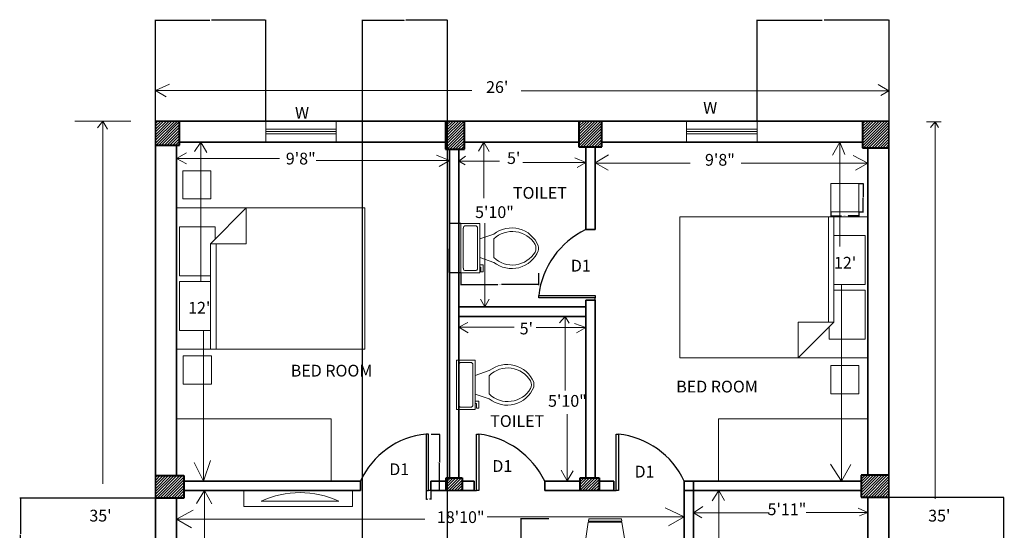
# Model space of a CAD drawing. Units: inches. Extents: x -34 to 385, y -422 to 64.
# Tile 3 of 3: x -34 to 385, y -153 to 64. Entities that reach past the tile are written whole.
import ezdxf

# ---------------------------------------------------------------- set-up
doc = ezdxf.new("R2010")
doc.units = ezdxf.units.IN
doc.header["$MEASUREMENT"] = 0
for name, color, linetype, lineweight in [('A-ANNO-DIMS', 2, 'Continuous', 13), ('A-ANNO-TEXT', 7, 'Continuous', 18), ('A-AREA-IDEN', 7, 'Continuous', 25), ('A-COLS', 1, 'Continuous', 40), ('A-COLS-PATT', 252, 'Continuous', 13), ('A-DOOR', 3, 'Continuous', 25), ('A-FLOR-CASE', 32, 'Continuous', 20), ('A-FLOR-FIXT', 9, 'Continuous', 18), ('A-FURN', 8, 'Continuous', 18), ('A-GLAZ', 4, 'Continuous', 18), ('A-WALL', 7, 'Continuous', 35)]:
    doc.layers.add(name, color=color, linetype=linetype, lineweight=lineweight)
doc.styles.get("Standard").update_dxf_attribs({"font": 'arial.ttf'})
doc.dimstyles.get("Standard").update_dxf_attribs({"dimtxt": 0.18, "dimasz": 0.18, "dimexe": 0.18, "dimexo": 0.0625, "dimgap": 0.09, "dimtad": 0, "dimtih": 1, "dimtoh": 1, "dimdec": 4, "dimzin": 0, "dimdsep": 46, "dimtxsty": 'Standard', "dimcen": 0.09, "dimadec": 0, "dimazin": 0, "dimtfac": 1, "dimtdec": 4, "dimtofl": 0, "dimtmove": 0, "dimatfit": 3, "dimfxl": 1, "dimtolj": 1, "dimtzin": 0, "dimarcsym": 0})

# ---------------------------------------------------------------- blocks, each defined once
blk = doc.blocks.new('Toilet - top')
for p, q in [((9.5, -6), (9.5, -2)), ((-8, -8.5), (-8, -8)), ((-7, -8), (-7, -9.5)), ((-4, -8), (-6, -14)), ((4, -8), (6, -14)), ((-10, -8.5), (-8, -8.5)), ((-10, -9.5), (-10, -8.5)), ((-7, -9.5), (-10, -9.5)), ((4, -14), (-4, -14))]:
    blk.add_line(p, q)
blk.add_lwpolyline([(10.5, -8), (10.5, 0), (-10.5, 0), (-10.5, -8)], close=True)
for points in [[(-9.5, -2), (-9.5, -6)], [(8.5, -1), (-8.5, -1)], [(-8.5, -7), (8.5, -7)]]:
    blk.add_lwpolyline(points)
for centre, radius, start, end in [((-8.62, -1.88), 0.884, 81.8699, 188.1301), ((8.62, -1.88), 0.884, 351.8699, 98.1301), ((-8.62, -6.12), 0.884, 171.8699, 278.1301), ((8.62, -6.12), 0.884, 261.8699, 8.1301), ((3.52, -21.58), 12.17, 141.4691, 247.9714), ((4.2, -21.82), 11.33, 136.3677, 238.9468), ((-3.52, -21.58), 12.17, 292.0284, 38.5307), ((-4.2, -21.82), 11.33, 301.053, 43.6321), ((0, -27.88), 4, 245.7318, 294.2682), ((0, -29), 4, 254.8605, 285.1395)]:
    blk.add_arc(centre, radius, start, end)
blk = doc.blocks.new('Bed - Queen')
for p, q in [((0, -80.00003), (0, 0)), ((0, 0), (59.99999, 0)), ((59.99999, 0), (59.99999, -80.00003)), ((7.99999, -1.2), (28.79998, -1.2)), ((7.99999, -14.4), (7.99999, -1.2)), ((28.79998, -1.2), (28.79998, -14.4)), ((31.19999, -1.2), (51.99999, -1.2)), ((31.19999, -14.4), (31.19999, -1.2)), ((51.99999, -1.2), (51.99999, -16.4)), ((0, -14.4), (44.8, -14.4)), ((59.99999, -29.6), (44.8, -14.4)), ((44.8, -14.4), (44.8, -29.6)), ((51.99999, -16.4), (46.79936, -16.4)), ((44.8, -16.8), (0, -16.8)), ((44.8, -29.6), (59.99999, -29.6)), ((59.99999, -80.00003), (0, -80.00003))]:
    blk.add_line(p, q)
blk = doc.blocks.new('Dining Set - 36 x 72 in.')
for p, q in [((-22.2343, 26.00059), (-23.4847, 17.99762)), ((-22.2304, 26), (-5.7608, 26)), ((-22, 27.5), (-22.1562, 26.50042)), ((-5.8416, 26.5), (-22.1534, 26.5)), ((-22, 27.5), (-6, 27.5)), ((-5.8437, 26.49966), (-6, 27.5)), ((-4.5152, 17.99762), (-5.7655, 25.99926)), ((5.7657, 26.00059), (4.5153, 17.99762)), ((5.7696, 26), (22.2392, 26)), ((6, 27.5), (5.8438, 26.50042)), ((22.1584, 26.5), (5.8466, 26.5)), ((6, 27.5), (22, 27.5)), ((22.1563, 26.49966), (22, 27.5)), ((23.4848, 17.99762), (22.2345, 25.99926)), ((36, 18), (-36, 18)), ((-36, 18), (-36, -18)), ((36, -18), (36, 18)), ((-45.5, 8), (-44.5004, 8.15617)), ((-45.5, 8), (-45.5, -8)), ((-44.5, -8.15843), (-44.5, 8.15338)), ((-44.0006, 8.23428), (-35.9976, 9.48474)), ((-44, 8.23041), (-44, -8.23915)), ((44.0006, 8.23428), (35.9976, 9.48474)), ((44, 8.23041), (44, -8.23915)), ((44.5, -8.15843), (44.5, 8.15338)), ((45.5, 8), (44.5005, 8.15617)), ((45.5, 8), (45.5, -8)), ((-44.4997, -8.15631), (-45.5, -8)), ((-35.9976, -9.48476), (-43.9993, -8.2345)), ((35.9976, -9.48476), (43.9993, -8.2345)), ((44.4997, -8.15631), (45.5, -8)), ((-36, -18), (36, -18)), ((-22.2343, -26.0006), (-23.4847, -17.99762)), ((-4.5152, -17.99762), (-5.7655, -25.99928)), ((5.7657, -26.0006), (4.5153, -17.99762)), ((23.4848, -17.99762), (22.2345, -25.99928)), ((-22.2304, -26), (-5.7608, -26)), ((-22, -27.5), (-22.1562, -26.50044)), ((-5.8416, -26.5), (-22.1534, -26.5)), ((-22, -27.5), (-6, -27.5)), ((-5.8437, -26.49967), (-6, -27.5)), ((5.7696, -26), (22.2392, -26)), ((6, -27.5), (5.8438, -26.50044)), ((22.1584, -26.5), (5.8466, -26.5)), ((6, -27.5), (22, -27.5)), ((22.1563, -26.49967), (22, -27.5))]:
    blk.add_line(p, q)
for points in [[(-36, 15), (-31.1772, 14.97754), (-26.8079, 14.91406), (-22.8538, 14.81543), (-19.276, 14.6875), (-16.0362, 14.53613), (-13.0957, 14.36718), (-10.4159, 14.18652), (-7.9583, 14), (-5.6904, 13.81315), (-3.6035, 13.63021), (-1.6954, 13.45508), (0.0365, 13.29166), (1.5945, 13.14388), (2.9811, 13.01562), (4.1988, 12.9108), (5.25, 12.83333), (6.1393, 12.78613), (6.8802, 12.76823), (7.4883, 12.77767), (7.9792, 12.8125), (8.3685, 12.87077), (8.6719, 12.95052), (8.9049, 13.0498), (9.0833, 13.16666), (9.2205, 13.29899), (9.3216, 13.44401), (9.3895, 13.59879), (9.4271, 13.76041), (9.4373, 13.92594), (9.4232, 14.09245), (9.3875, 14.257), (9.3333, 14.41666), (9.2638, 14.56917), (9.1836, 14.71484), (9.0975, 14.85465), (9.0104, 14.98958), (8.9272, 15.1206), (8.8529, 15.2487), (8.7922, 15.37483), (8.75, 15.5), (8.7305, 15.62467), (8.7344, 15.74739), (8.7617, 15.86621), (8.8125, 15.97916), (8.8867, 16.08431), (8.9844, 16.17968), (9.1055, 16.26334), (9.25, 16.33333), (9.4189, 16.38802), (9.6172, 16.42708), (9.8506, 16.45052), (10.125, 16.45833), (10.4463, 16.45052), (10.8203, 16.42708), (11.2529, 16.38802), (11.75, 16.33333), (12.3184, 16.26318), (12.9694, 16.17838), (13.7151, 16.07991), (14.5677, 15.96875), (15.5395, 15.84586), (16.6426, 15.71224), (17.8893, 15.56884), (19.2917, 15.41666), (20.859, 15.25667), (22.5879, 15.08984), (24.4721, 14.91715), (26.5052, 14.73958), (28.6809, 14.5581), (30.9929, 14.3737), (33.4347, 14.18733), (36, 14)], [(-36, 10), (-28.9766, 10.14274), (-23.1725, 10.20442), (-18.4241, 10.19775), (-14.5677, 10.13541), (-11.4399, 10.03011), (-8.877, 9.89453), (-6.7154, 9.74137), (-4.7917, 9.58333), (-2.9698, 9.43082), (-1.2246, 9.28515), (0.4415, 9.14534), (2.026, 9.01041), (3.5266, 8.87939), (4.9408, 8.7513), (6.266, 8.62516), (7.5, 8.5), (8.6411, 8.37549), (9.6914, 8.2539), (10.6538, 8.13818), (11.5312, 8.03125), (12.3267, 7.93603), (13.043, 7.85547), (13.6831, 7.79248), (14.25, 7.75), (14.7471, 7.7303), (15.1797, 7.73307), (15.5537, 7.75732), (15.875, 7.80208), (16.1494, 7.86637), (16.3828, 7.94922), (16.5811, 8.04964), (16.75, 8.16666), (16.8944, 8.29915), (17.0143, 8.44531), (17.1089, 8.60319), (17.1771, 8.77083), (17.218, 8.94629), (17.2305, 9.1276), (17.2137, 9.31282), (17.1667, 9.5), (17.0895, 9.6875), (16.987, 9.875), (16.8649, 10.0625), (16.7292, 10.25), (16.5856, 10.4375), (16.4401, 10.625), (16.2985, 10.8125), (16.1667, 11), (16.05, 11.18733), (15.9518, 11.3737), (15.8752, 11.5581), (15.8229, 11.73958), (15.798, 11.91715), (15.8034, 12.08984), (15.842, 12.25667), (15.9167, 12.41666), (16.0295, 12.56836), (16.1784, 12.70833), (16.3605, 12.83268), (16.5729, 12.9375), (16.8127, 13.01888), (17.0768, 13.07291), (17.3625, 13.0957), (17.6667, 13.08333), (17.9894, 13.03312), (18.3418, 12.94726), (18.7382, 12.82918), (19.1927, 12.68229), (19.7195, 12.51001), (20.3327, 12.31575), (21.0465, 12.10294), (21.875, 11.875), (22.8357, 11.63354), (23.959, 11.37304), (25.2786, 11.08618), (26.8282, 10.76562), (28.6414, 10.40405), (30.752, 9.99414), (33.1936, 9.52856), (36, 9)], [(-36, 5.5), (-30.7157, 5.3348), (-26.069, 5.20963), (-21.9946, 5.11767), (-18.4271, 5.05208), (-15.3009, 5.00602), (-12.5508, 4.97265), (-10.1112, 4.94515), (-7.9167, 4.91666), (-5.909, 4.88167), (-4.0586, 4.83984), (-2.3429, 4.79215), (-0.7396, 4.73958), (0.7739, 4.6831), (2.22, 4.6237), (3.6213, 4.56233), (5, 4.5), (6.373, 4.43782), (7.7344, 4.3776), (9.0723, 4.32129), (10.375, 4.27083), (11.6309, 4.22819), (12.8281, 4.19531), (13.9551, 4.17415), (15, 4.16666), (15.954, 4.17448), (16.819, 4.19791), (17.6001, 4.23698), (18.3021, 4.29166), (18.9299, 4.36198), (19.4883, 4.44791), (19.9823, 4.54948), (20.4167, 4.66666), (20.7969, 4.79899), (21.1302, 4.94401), (21.4245, 5.09879), (21.6875, 5.26041), (21.9271, 5.42594), (22.1511, 5.59245), (22.3672, 5.757), (22.5834, 5.91666), (22.8065, 6.06868), (23.0404, 6.21093), (23.2879, 6.34147), (23.5521, 6.45833), (23.8358, 6.55957), (24.142, 6.64323), (24.4735, 6.70735), (24.8334, 6.75), (25.2235, 6.76969), (25.642, 6.76692), (26.0858, 6.74267), (26.5521, 6.69791), (27.0379, 6.63362), (27.5404, 6.55078), (28.0565, 6.45036), (28.5834, 6.33333), (29.1242, 6.19987), (29.7071, 6.04687), (30.3661, 5.87044), (31.1354, 5.66666), (32.0493, 5.43164), (33.142, 5.16146), (34.4475, 4.85221), (36, 4.5)], [(-36, -1), (-30.7915, -0.6591), (-26.0195, -0.38216), (-21.6519, -0.16284), (-17.6563, 0.00521), (-14.0005, 0.12833), (-10.6523, 0.21289), (-7.5796, 0.26522), (-4.75, 0.29166), (-2.134, 0.29793), (0.2878, 0.28711), (2.5317, 0.26163), (4.6146, 0.22396), (6.5529, 0.17651), (8.3633, 0.12174), (10.0623, 0.06209), (11.6667, 0), (13.1899, -0.06201), (14.6341, -0.1211), (15.9982, -0.17432), (17.2813, -0.21875), (18.4823, -0.25147), (19.6003, -0.26953), (20.6343, -0.27002), (21.5834, -0.25), (22.4481, -0.20768), (23.2357, -0.14584), (23.9549, -0.06836), (24.6146, 0.02083), (25.2235, 0.11784), (25.7904, 0.21875), (26.3241, 0.31966), (26.8334, 0.41666), (27.3265, 0.50618), (27.8099, 0.58593), (28.2894, 0.65397), (28.7709, 0.70833), (29.2601, 0.74707), (29.763, 0.76823), (30.2855, 0.76985), (30.8334, 0.75), (31.4088, 0.70784), (31.9994, 0.64713), (32.589, 0.57275), (33.1615, 0.48958), (33.7008, 0.4025), (34.1908, 0.3164), (34.6153, 0.23616), (34.9584, 0.16666), (35.2099, 0.11165), (35.3848, 0.07031), (35.504, 0.04069), (35.5886, 0.02083), (35.6594, 0.00879), (35.7377, 0.0026), (35.8442, 0.00032), (36, 0)], [(-36, -6.5), (-27.1843, -6.31267), (-20.084, -6.1263), (-14.469, -5.9419), (-10.1094, -5.76042), (-6.7752, -5.58285), (-4.2363, -5.41016), (-2.2629, -5.24333), (-0.625, -5.08334), (0.8708, -4.93099), (2.2715, -4.78646), (3.5872, -4.64974), (4.8281, -4.52084), (6.0046, -4.39974), (7.127, -4.28646), (8.2053, -4.18099), (9.25, -4.08334), (10.2705, -3.99382), (11.2734, -3.91407), (12.2647, -3.84603), (13.25, -3.79167), (14.2354, -3.75293), (15.2266, -3.73177), (16.2295, -3.73015), (17.25, -3.75), (18.2912, -3.79248), (19.3451, -3.85547), (20.4009, -3.93604), (21.4479, -4.03125), (22.4754, -4.13819), (23.4727, -4.25391), (24.4289, -4.37549), (25.3334, -4.5), (26.1785, -4.62492), (26.9694, -4.74935), (27.7145, -4.87281), (28.4219, -4.99479), (29.1, -5.11483), (29.7572, -5.23242), (30.4016, -5.34709), (31.0417, -5.45834), (31.6837, -5.56437), (32.3262, -5.65821), (32.9658, -5.73153), (33.599, -5.77604), (34.2224, -5.78345), (34.8327, -5.74545), (35.4264, -5.65373), (36, -5.5)], [(-36, -10), (-26.4022, -9.81299), (-18.4675, -9.62891), (-11.9839, -9.45069), (-6.7396, -9.28125), (-2.5226, -9.12354), (0.8789, -8.98047), (3.6769, -8.85498), (6.0833, -8.75), (8.2767, -8.66765), (10.3021, -8.60677), (12.1712, -8.56543), (13.8958, -8.54167), (15.4876, -8.53353), (16.9583, -8.53907), (18.3197, -8.55632), (19.5834, -8.58334), (20.7616, -8.61841), (21.8685, -8.66081), (22.9188, -8.71004), (23.9271, -8.76563), (24.9081, -8.82707), (25.8763, -8.89388), (26.8465, -8.96558), (27.8334, -9.04167), (28.8474, -9.12118), (29.8828, -9.20117), (30.93, -9.27824), (31.9792, -9.34896), (33.0205, -9.40991), (34.0443, -9.45768), (35.0407, -9.48885), (36, -9.5)], [(-36, -14.5), (-30.0881, -14.33513), (-25.0332, -14.21224), (-20.7312, -14.12647), (-17.0781, -14.07292), (-13.97, -14.04671), (-11.3027, -14.04297), (-8.9724, -14.05681), (-6.875, -14.08334), (-4.9224, -14.11833), (-3.0905, -14.16016), (-1.3709, -14.20785), (0.2448, -14.26042), (1.7647, -14.3169), (3.1973, -14.3763), (4.5507, -14.43767), (5.8333, -14.5), (7.0554, -14.5621), (8.235, -14.62175), (9.3922, -14.67652), (10.5469, -14.72396), (11.7192, -14.76164), (12.929, -14.78711), (14.1965, -14.79794), (15.5417, -14.79167), (16.9933, -14.76424), (18.6152, -14.70508), (20.4804, -14.60197), (22.6615, -14.44271), (25.2312, -14.21509), (28.2624, -13.9069), (31.8277, -13.50594), (36, -13)]]:
    blk.add_lwpolyline(points)
blk = doc.blocks.new('WIN-30IN-9IN-WALL')
for p, q in [((0, 9), (0, 0)), ((30, 9), (30, 0)), ((0, 5.5), (30, 5.5)), ((0, 4.5), (30, 4.5)), ((0, 3.5), (30, 3.5))]:
    blk.add_line(p, q)
blk = doc.blocks.new('DOOR-LEAF-24IN')
for p, q in [((1, 24), (0, 24)), ((0, 24), (0, 0)), ((1, 0), (1, 24)), ((0, 0), (1, 0)), ((2, 0), (1, 0))]:
    blk.add_line(p, q)
blk = doc.blocks.new('NIGHTSTAND-12IN')
blk.add_lwpolyline([(12, 0), (0, 0), (0, 12), (12, 12)], close=True)
blk = doc.blocks.new('*D12')
at = {"layer": 'A-ANNO-DIMS', "color": 0, "lineweight": -2, "transparency": 16777216}
for p, q in [((141.47, -112.14), (145.18, -112.14)), ((145, -112.32), (145, -123.96)), ((145, -135.96), (145, -124.32)), ((141.47, -136.14), (145.18, -136.14))]:
    blk.add_line(p, q, dxfattribs=at)
at = {"layer": 'A-ANNO-DIMS', "color": 0, "transparency": 16777216}
for points in [[(144.97, -112.32), (145.03, -112.32), (145, -112.14)], [(144.97, -135.96), (145.03, -135.96), (145, -136.14)]]:
    blk.add_solid(points, dxfattribs=at)
at = {"layer": 'Defpoints', "color": 0, "transparency": 16777216}
for p in [(141.4, -112.14), (145, -112.14), (141.4, -136.14)]:
    blk.add_point(p, dxfattribs=at)
at = {"layer": 'A-ANNO-DIMS', "color": 0, "transparency": 16777216, "insert": (145, -124.14), "char_height": 0.18, "attachment_point": 5}
blk.add_mtext('\\A1;LEAF 24 TYP.', dxfattribs=at)
blk = doc.blocks.new('*D13')
at = {"layer": 'A-ANNO-DIMS', "color": 0, "lineweight": -2, "transparency": 16777216}
for p, q in [((139.4, -136.21), (139.4, -139.92)), ((141.4, -136.21), (141.4, -139.92)), ((139.58, -139.74), (139.94, -139.74)), ((141.22, -139.74), (140.86, -139.74))]:
    blk.add_line(p, q, dxfattribs=at)
at = {"layer": 'A-ANNO-DIMS', "color": 0, "transparency": 16777216}
for points in [[(139.58, -139.71), (139.58, -139.77), (139.4, -139.74)], [(141.22, -139.71), (141.22, -139.77), (141.4, -139.74)]]:
    blk.add_solid(points, dxfattribs=at)
at = {"layer": 'Defpoints', "color": 0, "transparency": 16777216}
for p in [(139.4, -136.14), (141.4, -136.14), (141.4, -139.74)]:
    blk.add_point(p, dxfattribs=at)
at = {"layer": 'A-ANNO-DIMS', "color": 0, "transparency": 16777216, "insert": (140.4, -139.74), "char_height": 0.18, "attachment_point": 5}
blk.add_mtext('\\A1;2 TYP.', dxfattribs=at)
blk = doc.blocks.new('*D16')
at = {"layer": 'A-ANNO-DIMS', "color": 0, "lineweight": -2, "transparency": 16777216}
for p, q in [((154.2, -43.76), (154.2, -48.83)), ((187.24, -43.76), (187.24, -48.83)), ((154.38, -48.65), (169.94, -48.65)), ((187.06, -48.65), (171.5, -48.65))]:
    blk.add_line(p, q, dxfattribs=at)
at = {"layer": 'A-ANNO-DIMS', "color": 0, "transparency": 16777216}
for points in [[(154.38, -48.62), (154.38, -48.68), (154.2, -48.65)], [(187.06, -48.62), (187.06, -48.68), (187.24, -48.65)]]:
    blk.add_solid(points, dxfattribs=at)
at = {"layer": 'Defpoints', "color": 0, "transparency": 16777216}
for p in [(154.2, -43.69), (187.24, -43.69), (154.2, -48.65)]:
    blk.add_point(p, dxfattribs=at)
at = {"layer": 'A-ANNO-DIMS', "color": 0, "transparency": 16777216, "insert": (170.72, -48.65), "char_height": 0.18, "attachment_point": 5}
blk.add_mtext('\\A1;WC 33 TYP.', dxfattribs=at)
blk = doc.blocks.new('*D17')
at = {"layer": 'A-ANNO-DIMS', "color": 0, "lineweight": -2, "transparency": 16777216}
for p, q in [((154.13, -22.69), (149.06, -22.69)), ((149.24, -22.87), (149.24, -33.01)), ((149.24, -43.51), (149.24, -33.38)), ((154.13, -43.69), (149.06, -43.69))]:
    blk.add_line(p, q, dxfattribs=at)
at = {"layer": 'A-ANNO-DIMS', "color": 0, "transparency": 16777216}
for points in [[(149.21, -22.87), (149.27, -22.87), (149.24, -22.69)], [(149.21, -43.51), (149.27, -43.51), (149.24, -43.69)]]:
    blk.add_solid(points, dxfattribs=at)
at = {"layer": 'Defpoints', "color": 0, "transparency": 16777216}
for p in [(149.24, -22.69), (154.2, -22.69), (154.2, -43.69)]:
    blk.add_point(p, dxfattribs=at)
at = {"layer": 'A-ANNO-DIMS', "color": 0, "transparency": 16777216, "insert": (149.24, -33.19), "char_height": 0.18, "attachment_point": 5}
blk.add_mtext('\\A1;21 TYP.', dxfattribs=at)
blk = doc.blocks.new('*D18')
at = {"layer": 'A-ANNO-DIMS', "color": 0, "lineweight": -2, "transparency": 16777216}
for p, q in [((311.45, -17.73), (311.45, -19.64)), ((311.63, -19.46), (316.08, -19.46)), ((323.27, -19.46), (318.83, -19.46)), ((323.45, -17.73), (323.45, -19.64))]:
    blk.add_line(p, q, dxfattribs=at)
at = {"layer": 'A-ANNO-DIMS', "color": 0, "transparency": 16777216}
for points in [[(311.63, -19.43), (311.63, -19.49), (311.45, -19.46)], [(323.27, -19.43), (323.27, -19.49), (323.45, -19.46)]]:
    blk.add_solid(points, dxfattribs=at)
at = {"layer": 'Defpoints', "color": 0, "transparency": 16777216}
for p in [(311.45, -17.66), (323.45, -17.66), (323.45, -19.46)]:
    blk.add_point(p, dxfattribs=at)
at = {"layer": 'A-ANNO-DIMS', "color": 0, "transparency": 16777216, "insert": (317.45, -19.46), "char_height": 0.18, "attachment_point": 5}
blk.add_mtext('\\A1;NIGHTSTAND 12 TYP.', dxfattribs=at)
blk = doc.blocks.new('*D19')
at = {"layer": 'A-ANNO-DIMS', "color": 0, "lineweight": -2, "transparency": 16777216}
for p, q in [((323.51, -5.66), (325.43, -5.66)), ((325.25, -5.84), (325.25, -11.48)), ((325.25, -17.48), (325.25, -11.84)), ((323.51, -17.66), (325.43, -17.66))]:
    blk.add_line(p, q, dxfattribs=at)
at = {"layer": 'A-ANNO-DIMS', "color": 0, "transparency": 16777216}
for points in [[(325.22, -5.84), (325.28, -5.84), (325.25, -5.66)], [(325.22, -17.48), (325.28, -17.48), (325.25, -17.66)]]:
    blk.add_solid(points, dxfattribs=at)
at = {"layer": 'Defpoints', "color": 0, "transparency": 16777216}
for p in [(323.45, -5.66), (325.25, -5.66), (323.45, -17.66)]:
    blk.add_point(p, dxfattribs=at)
at = {"layer": 'A-ANNO-DIMS', "color": 0, "transparency": 16777216, "insert": (325.25, -11.66), "char_height": 0.18, "attachment_point": 5}
blk.add_mtext('\\A1;12 TYP.', dxfattribs=at)
blk = doc.blocks.new('*D32')
at = {"layer": 'A-ANNO-DIMS', "color": 0, "lineweight": -2, "transparency": 16777216}
for p, q in [((191.51, -148.21), (179.52, -148.21)), ((179.7, -148.39), (179.7, -187.61)), ((179.7, -227.2), (179.7, -187.98)), ((191.51, -227.38), (179.52, -227.38))]:
    blk.add_line(p, q, dxfattribs=at)
at = {"layer": 'A-ANNO-DIMS', "color": 0, "transparency": 16777216}
for points in [[(179.67, -148.39), (179.73, -148.39), (179.7, -148.21)], [(179.67, -227.2), (179.73, -227.2), (179.7, -227.38)]]:
    blk.add_solid(points, dxfattribs=at)
at = {"layer": 'Defpoints', "color": 0, "transparency": 16777216}
for p in [(191.58, -148.21), (179.7, -227.38), (191.58, -227.38)]:
    blk.add_point(p, dxfattribs=at)
at = {"layer": 'A-ANNO-DIMS', "color": 0, "transparency": 16777216, "insert": (179.7, -187.79), "char_height": 0.18, "attachment_point": 5}
blk.add_mtext('\\A1;DINING SET 79', dxfattribs=at)
blk = doc.blocks.new('*D34')
at = {"layer": 'A-ANNO-DIMS', "color": 0, "lineweight": -2, "transparency": 16777216}
for p, q in [((24.26, 20.92), (24.26, 63.89)), ((24.44, 63.71), (47.38, 63.71)), ((70.97, 63.71), (48.03, 63.71)), ((71.15, 20.92), (71.15, 63.89))]:
    blk.add_line(p, q, dxfattribs=at)
at = {"layer": 'A-ANNO-DIMS', "color": 0, "transparency": 16777216}
for points in [[(24.44, 63.74), (24.44, 63.68), (24.26, 63.71)], [(70.97, 63.74), (70.97, 63.68), (71.15, 63.71)]]:
    blk.add_solid(points, dxfattribs=at)
at = {"layer": 'Defpoints', "color": 0, "transparency": 16777216}
for p in [(71.15, 63.71), (24.26, 20.86), (71.15, 20.86)]:
    blk.add_point(p, dxfattribs=at)
at = {"layer": 'A-ANNO-DIMS', "color": 0, "transparency": 16777216, "insert": (47.7, 63.71), "char_height": 0.18, "attachment_point": 5}
blk.add_mtext('\\A1;46.9', dxfattribs=at)
blk = doc.blocks.new('*D35')
at = {"layer": 'A-ANNO-DIMS', "color": 0, "lineweight": -2, "transparency": 16777216}
for p, q in [((280.19, 20.92), (280.19, 63.89)), ((280.37, 63.71), (307.83, 63.71)), ((336.08, 63.71), (308.62, 63.71)), ((336.26, 20.92), (336.26, 63.89))]:
    blk.add_line(p, q, dxfattribs=at)
at = {"layer": 'A-ANNO-DIMS', "color": 0, "transparency": 16777216}
for points in [[(280.37, 63.74), (280.37, 63.68), (280.19, 63.71)], [(336.08, 63.74), (336.08, 63.68), (336.26, 63.71)]]:
    blk.add_solid(points, dxfattribs=at)
at = {"layer": 'Defpoints', "color": 0, "transparency": 16777216}
for p in [(336.26, 63.71), (280.19, 20.86), (336.26, 20.86)]:
    blk.add_point(p, dxfattribs=at)
at = {"layer": 'A-ANNO-DIMS', "color": 0, "transparency": 16777216, "insert": (308.22, 63.71), "char_height": 0.18, "attachment_point": 5}
blk.add_mtext('\\A1;56.07', dxfattribs=at)
blk = doc.blocks.new('*D36')
at = {"layer": 'A-ANNO-DIMS', "color": 0, "lineweight": -2, "transparency": 16777216}
for p, q in [((24.19, -139.38), (-33.38, -139.38)), ((-33.2, -139.56), (-33.2, -154.58)), ((-33.2, -169.95), (-33.2, -154.94)), ((24.19, -170.13), (-33.38, -170.13))]:
    blk.add_line(p, q, dxfattribs=at)
at = {"layer": 'A-ANNO-DIMS', "color": 0, "transparency": 16777216}
for points in [[(-33.23, -139.56), (-33.17, -139.56), (-33.2, -139.38)], [(-33.23, -169.95), (-33.17, -169.95), (-33.2, -170.13)]]:
    blk.add_solid(points, dxfattribs=at)
at = {"layer": 'Defpoints', "color": 0, "transparency": 16777216}
for p in [(24.26, -139.38), (-33.2, -170.13), (24.26, -170.13)]:
    blk.add_point(p, dxfattribs=at)
at = {"layer": 'A-ANNO-DIMS', "color": 0, "transparency": 16777216, "insert": (-33.2, -154.76), "char_height": 0.18, "attachment_point": 5}
blk.add_mtext('\\A1;30.75', dxfattribs=at)
blk = doc.blocks.new('*D37')
at = {"layer": 'A-ANNO-DIMS', "color": 0, "lineweight": -2, "transparency": 16777216}
for p, q in [((336.32, -138.89), (385.11, -138.89)), ((384.93, -139.07), (384.93, -156.71)), ((384.93, -174.71), (384.93, -157.07)), ((336.32, -174.89), (385.11, -174.89))]:
    blk.add_line(p, q, dxfattribs=at)
at = {"layer": 'A-ANNO-DIMS', "color": 0, "transparency": 16777216}
for points in [[(384.9, -139.07), (384.96, -139.07), (384.93, -138.89)], [(384.9, -174.71), (384.96, -174.71), (384.93, -174.89)]]:
    blk.add_solid(points, dxfattribs=at)
at = {"layer": 'Defpoints', "color": 0, "transparency": 16777216}
for p in [(336.26, -138.89), (336.26, -174.89), (384.93, -174.89)]:
    blk.add_point(p, dxfattribs=at)
at = {"layer": 'A-ANNO-DIMS', "color": 0, "transparency": 16777216, "insert": (384.93, -156.89), "char_height": 0.18, "attachment_point": 5}
blk.add_mtext('\\A1;35.995', dxfattribs=at)
blk = doc.blocks.new('*D39')
at = {"layer": 'A-ANNO-DIMS', "color": 0, "lineweight": -2, "transparency": 16777216}
for p, q in [((112.34, -351.08), (112.34, 63.89)), ((112.52, 63.71), (129.99, 63.71)), ((148.25, 63.71), (130.78, 63.71)), ((148.43, -351.08), (148.43, 63.89))]:
    blk.add_line(p, q, dxfattribs=at)
at = {"layer": 'A-ANNO-DIMS', "color": 0, "transparency": 16777216}
for points in [[(112.52, 63.74), (112.52, 63.68), (112.34, 63.71)], [(148.25, 63.74), (148.25, 63.68), (148.43, 63.71)]]:
    blk.add_solid(points, dxfattribs=at)
at = {"layer": 'Defpoints', "color": 0, "transparency": 16777216}
for p in [(148.43, 63.71), (112.34, -351.14), (148.43, -351.14)]:
    blk.add_point(p, dxfattribs=at)
at = {"layer": 'A-ANNO-DIMS', "color": 0, "transparency": 16777216, "insert": (130.38, 63.71), "char_height": 0.18, "attachment_point": 5}
blk.add_mtext('\\A1;36.09', dxfattribs=at)

msp = doc.modelspace()

# ---------------------------------------------------------------- hatches: boundary and pattern name
at = {"layer": 'A-COLS-PATT'}
h = msp.add_hatch(dxfattribs=at)
h.set_pattern_fill('ANSI31', color=256, scale=6.7)
h.set_pattern_definition([(45, (-1587.6103, -800.894), (-0.59220193, 0.59220193), [])])
h.paths.add_polyline_path([(34.5325, 20.857), (24.2567, 20.857), (24.2567, 10.5552), (34.5325, 10.5552)])
h.paths.add_polyline_path([(155.6882, 20.857), (147.6505, 20.857), (147.6505, 8.8355), (155.6882, 8.8355)])
h.paths.add_polyline_path([(214.1102, 20.857), (204.3358, 20.857), (204.3358, 9.8804), (214.1102, 9.8804)])
h.paths.add_polyline_path([(336.2567, 20.857), (324.9664, 20.857), (324.9664, 9.4113), (336.2567, 9.4113)])
h.paths.add_polyline_path([(336.2567, -129.6656), (324.4892, -129.6656), (324.4892, -138.8931), (336.2567, -138.8931)])
h.paths.add_polyline_path([(212.9763, -130.7216), (204.8831, -130.7216), (204.8831, -136.143), (212.9763, -136.143)])
h.paths.add_polyline_path([(154.6774, -130.7571), (147.9004, -130.7571), (147.9004, -136.143), (154.6774, -136.143)])
h.paths.add_polyline_path([(36.3503, -129.7825), (24.2567, -129.7825), (24.2567, -139.3836), (36.3503, -139.3836)])
h.paths.add_polyline_path([(35.9496, -230.9729), (24.2567, -230.9729), (24.2567, -238.1404), (35.9496, -238.1404)])
h.paths.add_polyline_path([(153.2567, -232.143), (148.2796, -232.143), (148.2796, -237.1221), (148.2796, -237.5145), (153.2567, -237.5145)])
h.paths.add_polyline_path([(212.7, -232.143), (207.2567, -232.143), (207.2567, -238.4312), (212.7, -238.4312)])
h.paths.add_polyline_path([(336.2567, -230.9985), (325.0216, -230.9985), (325.0216, -236.8618), (336.2567, -236.8618)])
h.paths.add_polyline_path([(34.6412, -348.0183), (24.2567, -348.0183), (24.2567, -355.143), (33.2567, -355.143), (34.6412, -355.143)])
h.paths.add_polyline_path([(35.0834, -388.1327), (24.2567, -388.1327), (24.2567, -399.143), (35.0834, -399.143)])
h.paths.add_polyline_path([(156.485, -388.1078), (149.2567, -388.1078), (149.2567, -390.143), (149.2567, -399.143), (156.485, -399.143)])
h.paths.add_polyline_path([(153.2567, -351.143), (148.4284, -351.143), (148.4284, -355.9617), (153.2567, -355.9617)])
h.paths.add_polyline_path([(211.2567, -390.143), (211.2567, -388.2391), (204.1967, -388.2391), (204.1967, -399.143), (211.2567, -399.143)])
h.paths.add_polyline_path([(213.2403, -351.143), (207.2567, -351.143), (207.2567, -356.6203), (213.2403, -356.6203)])
h.paths.add_polyline_path([(336.2567, -347.847), (325.718, -347.847), (325.718, -355.143), (327.2567, -355.143), (336.2567, -355.143)])
h.paths.add_polyline_path([(336.2567, -387.9228), (324.3995, -387.9228), (324.3995, -399.143), (336.2567, -399.143)])

# ---------------------------------------------------------------- linework, layer by layer
at = {"layer": 'A-ANNO-DIMS'}
for p, q in [((24.2567, 26.3154), (24.2567, 41.212)), ((336.2567, 33.7164), (336.2567, 39.4845)), ((30.1453, 36.5651), (24.2567, 33.7637)), ((24.2567, 33.7637), (158.7619, 33.7637)), ((24.2567, 33.7637), (28.8125, 31.1334)), ((179.8418, 33.7164), (336.2567, 33.7164)), ((331.5997, 36.4357), (336.2567, 33.7164)), ((336.2567, 33.7164), (332.7441, 31.6884)), ((336.2567, 33.7164), (336.2567, 27.6379)), ((13.7174, 20.857), (-10.0426, 20.857)), ((-0.4701, 17.9685), (1.8374, 20.857)), ((1.8374, 20.857), (1.8374, -133.3116)), ((1.8374, 20.857), (3.8184, 17.4258)), ((355.9176, 20.488), (352.2699, 20.488)), ((353.9558, 18.0485), (355.9176, 20.488)), ((355.9176, -139.6024), (355.9176, 20.488)), ((355.9176, 20.488), (358.5007, 20.488)), ((355.9176, 20.488), (357.2812, 18.1263)), ((40.7996, 7.8744), (43.607, 11.857)), ((43.607, 11.857), (43.607, -29.3761)), ((43.607, 11.857), (46.141, 7.4679)), ((161.7047, 8.0777), (163.9732, 11.857)), ((163.9732, 11.857), (163.9732, -11.858)), ((163.9732, 11.857), (166.2386, 7.9332)), ((312.1846, 6.3444), (315.4056, 11.857)), ((315.4056, 11.857), (315.4056, -32.4792)), ((315.4056, 11.857), (317.5145, 6.6321)), ((37.4059, 7.3458), (33.2567, 5.0005)), ((77.0001, 5.0005), (33.2567, 5.0005)), ((33.2567, 5.0005), (37.3815, 2.6191)), ((143.8179, 6.4124), (149.2567, 4.0942)), ((156.1052, 5.9612), (153.2567, 3.8565)), ((202.6804, 5.1951), (207.2567, 3.1751)), ((216.9389, 6.4197), (211.2567, 3.1391)), ((321.02, 6.1436), (327.2567, 2.9646)), ((92.5567, 4.0942), (149.2567, 4.0942)), ((149.2567, 4.0942), (144.887, 1.5714)), ((153.2567, 3.8565), (170.6177, 3.8565)), ((153.2567, 3.8565), (155.9483, 2.3025)), ((180.5086, 3.1751), (207.2567, 3.1751)), ((207.2567, 3.1751), (203.6563, 1.0964)), ((211.2567, 3.1391), (216.7931, -0.0574)), ((211.2567, 2.9646), (251.7319, 2.9646)), ((273.3457, 2.9646), (327.2567, 2.9646)), ((327.2567, 2.9646), (321.978, -0.083)), ((164.3173, -22.5122), (164.3173, -58.143)), ((43.607, -29.3761), (43.607, -47.2964)), ((315.9883, -48.5998), (315.9883, -132.143)), ((162.5127, -54.8117), (164.3173, -58.143)), ((164.3173, -58.143), (166.192, -54.8959)), ((164.3173, -58.143), (164.3173, -58.143)), ((196.1452, -64.91), (198.5473, -62.143)), ((198.5473, -62.143), (198.5473, -93.6636)), ((198.5473, -62.143), (200.2444, -65.0824)), ((157.0922, -64.7268), (153.2567, -66.7706)), ((153.2567, -66.7706), (176.8086, -66.7706)), ((153.2567, -66.7706), (157.2866, -69.0972)), ((186.1358, -66.8802), (207.2567, -66.8802)), ((202.4775, -65.1389), (207.2567, -66.8802)), ((207.2567, -66.8802), (203.3936, -69.1106)), ((44.664, -68.0964), (44.664, -132.143)), ((199.4286, -103.6991), (199.4286, -132.143)), ((40.6761, -124.2728), (44.664, -132.143)), ((44.664, -132.143), (47.6185, -123.3413)), ((311.322, -124.9355), (315.9883, -132.143)), ((315.9883, -132.143), (320.0759, -125.0632)), ((196.8102, -127.4379), (199.4286, -131.9731)), ((199.4286, -131.9731), (201.8615, -127.7592)), ((41.6941, -141.6629), (45.0444, -136.143)), ((45.0444, -136.143), (45.0444, -173.7502)), ((45.0444, -136.143), (48.2884, -141.7618)), ((261.0652, -140.5305), (263.8812, -136.143)), ((263.8812, -136.143), (263.8812, -186.9196)), ((263.8812, -136.143), (266.2842, -140.3051)), ((40.2666, -144.4566), (33.2567, -148.3057)), ((241.1179, -143.4254), (249.1677, -147.2714)), ((257.1238, -142.8438), (253.1677, -145.6416)), ((253.1677, -145.6416), (285.3097, -145.6416)), ((253.1677, -145.6416), (256.6798, -147.6693)), ((301.0775, -145.501), (327.2567, -145.501)), ((323.1927, -143.5724), (327.2567, -145.501)), ((327.2567, -145.501), (323.6788, -146.9366)), ((138.8592, -148.3057), (33.2567, -148.3057)), ((33.2567, -148.3057), (39.5026, -151.9118)), ((165.3148, -147.2714), (249.1677, -147.2714)), ((249.1677, -147.2714), (242.5285, -151.1045))]:
    msp.add_line(p, q, dxfattribs=at)
at = {"layer": 'A-COLS'}
for p, q in [((34.5325, 10.5552), (34.5325, 20.857)), ((147.6505, 20.857), (147.6505, 8.8355)), ((155.6882, 8.8355), (155.6882, 20.857)), ((204.3358, 20.857), (204.3358, 9.8804)), ((214.1102, 9.8804), (214.1102, 20.857)), ((324.9664, 20.857), (324.9664, 9.4113)), ((24.2567, 10.5552), (34.5325, 10.5552)), ((147.6505, 8.8355), (155.6882, 8.8355)), ((204.3358, 9.8804), (214.1102, 9.8804)), ((324.9664, 9.4113), (336.2567, 9.4113)), ((24.2567, -129.7825), (36.3503, -129.7825)), ((36.3503, -129.7825), (36.3503, -139.3836)), ((336.2567, -129.6656), (324.4892, -129.6656)), ((324.4892, -129.6656), (324.4892, -138.8931)), ((147.9004, -136.143), (147.9004, -130.7571)), ((147.9004, -130.7571), (154.6774, -130.7571)), ((154.6774, -130.7571), (154.6774, -136.143)), ((204.8831, -136.143), (204.8831, -130.7216)), ((204.8831, -130.7216), (212.9763, -130.7216)), ((212.9763, -130.7216), (212.9763, -136.143)), ((36.3503, -139.3836), (24.2567, -139.3836)), ((324.4892, -138.8931), (336.2567, -138.8931))]:
    msp.add_line(p, q, dxfattribs=at)
at = {"layer": 'A-DOOR'}
for centre, radius, start, end in [((222.7478, -57.4604), 35.7397, 115.686269, 173.238375), ((142.8752, -146.6041), 34.6355, 95.753529, 155.321827), ((157.5074, -147.7789), 35.8958, 25.823004, 83.10164), ((217.3821, -147.0427), 35.1044, 25.115226, 83.809418)]:
    msp.add_arc(centre, radius, start, end, dxfattribs=at)
at = {"layer": 'A-FLOR-CASE'}
for p, q in [((33.2567, -105.6851), (98.9803, -105.6851)), ((98.9803, -105.6851), (98.9803, -132.143)), ((327.2567, -105.6124), (263.7495, -105.6124)), ((263.7495, -105.6124), (263.7495, -132.143)), ((61.7676, -136.143), (61.7676, -142.8802)), ((108.1248, -142.8802), (108.1248, -136.143)), ((69.2031, -140.588), (102.2499, -140.588)), ((61.7676, -142.8802), (108.1248, -142.8802))]:
    msp.add_line(p, q, dxfattribs=at)
msp.add_arc((85.7265, -176.9686), 39.9571, 65.573339, 114.426661, dxfattribs=at)
at = {"layer": 'A-WALL'}
for p, q in [((33.2567, -129.7825), (33.2567, 10.5552)), ((34.5325, 11.857), (147.6505, 11.857)), ((149.2567, -130.7571), (149.2567, 8.8355)), ((153.2567, -130.7571), (153.2567, 8.8355)), ((155.6882, 11.857), (204.3358, 11.857)), ((207.2567, 9.8804), (207.2567, -25.2524)), ((211.2567, 9.8804), (211.2567, -25.2524)), ((214.1102, 11.857), (324.9664, 11.857)), ((327.2567, 9.4113), (327.2567, -129.6656)), ((207.2567, -25.2524), (211.2567, -25.2524)), ((207.2567, -58.143), (153.2567, -58.143)), ((207.2567, -55.2524), (211.2567, -55.2524)), ((207.2567, -55.2524), (207.2567, -130.7216)), ((211.2567, -55.2524), (211.2567, -130.7216)), ((153.2567, -62.143), (207.2567, -62.143)), ((36.3503, -132.143), (111.403, -132.143)), ((111.403, -136.143), (111.403, -132.143)), ((141.403, -136.143), (141.403, -132.143)), ((141.403, -132.143), (147.9004, -132.143)), ((154.6774, -132.143), (159.8188, -132.143)), ((159.8188, -132.143), (159.8188, -136.143)), ((189.8188, -132.143), (189.8188, -136.143)), ((189.8188, -132.143), (204.8831, -132.143)), ((212.9763, -132.143), (219.1677, -132.143)), ((219.1677, -132.143), (219.1677, -136.143)), ((249.1677, -132.143), (249.1677, -136.143)), ((249.1677, -132.143), (324.4892, -132.143)), ((253.1677, -196.8987), (253.1677, -132.143)), ((36.3503, -136.143), (111.403, -136.143)), ((141.403, -136.143), (159.8188, -136.143)), ((189.8188, -136.143), (219.1677, -136.143)), ((249.1677, -136.143), (324.4892, -136.143)), ((249.1677, -136.143), (249.1677, -196.8987)), ((33.2567, -230.9729), (33.2567, -139.3836)), ((327.2567, -138.8931), (327.2567, -230.9985))]:
    msp.add_line(p, q, dxfattribs=at)
msp.add_lwpolyline([(24.2567, 20.857), (336.2567, 20.857), (336.2567, -399.143), (24.2567, -399.143)], close=True, dxfattribs=at)

# ---------------------------------------------------------------- block references
at = {"layer": 'A-DOOR', "extrusion": (0, 0, -1), "zscale": -1, "rotation": 269.9999999999999}
msp.add_blockref('DOOR-LEAF-24IN', (-211.2567, -53.2524), dxfattribs=at)
at = {"layer": 'A-DOOR'}
msp.add_blockref('DOOR-LEAF-24IN', (139.403, -136.143), dxfattribs=at)
at = {"layer": 'A-DOOR', "extrusion": (0, 0, -1), "zscale": -1}
for p in [(-161.8188, -136.143), (-221.1676, -136.143)]:
    msp.add_blockref('DOOR-LEAF-24IN', p, dxfattribs=at)
at = {"layer": 'A-FLOR-FIXT', "rotation": 90}
for p in [(154.1958, -33.195), (152.2567, -91.1922)]:
    msp.add_blockref('Toilet - top', p, dxfattribs=at)
at = {"layer": 'A-FURN'}
for p in [(35.8296, -12.2578), (311.451, -17.664), (36.0404, -90.9546), (311.451, -95.0154)]:
    msp.add_blockref('NIGHTSTAND-12IN', p, dxfattribs=at)
for p, rotation in [((33.2567, -76.0964), 90), ((327.2567, -19.7998), 270)]:
    msp.add_blockref('Bed - Queen', p, dxfattribs=dict(at, rotation=rotation))
at = {"layer": 'A-FURN', "xscale": 0.8699120916390469, "yscale": 0.8699120916390469, "zscale": 0.8699120916390469, "rotation": 270}
msp.add_blockref('Dining Set - 36 x 72 in.', (215.499, -187.7941), dxfattribs=at)
at = {"layer": 'A-GLAZ'}
for p in [(71.152, 11.857), (250.1865, 11.857)]:
    msp.add_blockref('WIN-30IN-9IN-WALL', p, dxfattribs=at)

# ---------------------------------------------------------------- texts
at = {"layer": 'A-ANNO-DIMS', "char_height": 5, "attachment_point": 1}
for s, width, insert in [("26'", 22.71965, (164.8865, 37.7838)), ('9\'8"', 24.448319, (79.6878, 7.3844)), ("5'", 11.606778, (173.7798, 7.6085)), ('9\'8"', 1.234763, (257.9907, 6.8685)), ('5\'10"', 8.060841, (160.1909, -15.3554)), ("12'", 20.474628, (312.8567, -36.8597)), ("12'", 20.474628, (38.1546, -55.9789)), ("5'", 11.606778, (179.1565, -64.7888)), ('5\'10"', 8.060841, (191.2288, -95.5419)), ('5\'11"', 13.587919, (284.5966, -141.5987)), ("35'", 24.436189, (-3.8628, -144.2994)), ('18\'10"', 53.864306, (143.9518, -144.9337)), ("35'", 24.436189, (352.9233, -144.2994))]:
    msp.add_mtext_dynamic_manual_height_columns(s, width=width, gutter_width=25, heights=[0], dxfattribs=dict(at, insert=insert))
at = {"layer": 'A-ANNO-TEXT', "char_height": 5, "attachment_point": 1}
for s, width, insert in [('W', 4.868686, (83.5943, 26.8584)), ('W', 12.382851, (257.216, 28.9816)), ('D1', 13.576949, (200.9212, -38.1055)), ('D1', 11.147616, (123.6934, -124.583)), ('D1', 11.147616, (167.5461, -123.2176)), ('D1', 11.147616, (228.0258, -125.5933))]:
    msp.add_mtext_dynamic_manual_height_columns(s, width=width, gutter_width=25, heights=[0], dxfattribs=dict(at, insert=insert))
at = {"layer": 'A-AREA-IDEN', "char_height": 5, "attachment_point": 1}
for s, width, insert in [('TOILET', 27.75682, (176.306, -7.1677)), ('BED ROOM', 39.759385, (81.7891, -82.7019)), ('BED ROOM', 39.759385, (245.7456, -89.4648)), ('TOILET', 27.75682, (166.6465, -104.1149))]:
    msp.add_mtext_dynamic_manual_height_columns(s, width=width, gutter_width=25, heights=[0], dxfattribs=dict(at, insert=insert))

# ---------------------------------------------------------------- dimensions: what is measured, and where the dimension line sits
at = {"layer": 'A-ANNO-DIMS'}
for base, p1, p2, override, picture, middle in [((71.1521, 63.712), (24.2567, 20.857), (71.1521, 20.857), {"dimdec": 1, "dimlfac": 1, "dimrnd": 0, "dimzin": 0, "dimdsep": 46, "dimlunit": 2}, '*D34', (47.7044, 63.712)), ((148.4284, 63.712), (112.3403, -351.143), (148.4284, -351.143), {"dimdec": 2, "dimlfac": 1, "dimrnd": 0, "dimzin": 0, "dimdsep": 46, "dimlunit": 2}, '*D39', (130.3844, 63.712)), ((336.2567, 63.712), (280.1866, 20.857), (336.2567, 20.857), {"dimdec": 2, "dimlfac": 1, "dimrnd": 0, "dimzin": 0, "dimdsep": 46, "dimlunit": 2}, '*D35', (308.2217, 63.712))]:
    dim = msp.add_linear_dim(base=base, p1=p1, p2=p2, dimstyle='Standard', override=override, dxfattribs=at)
    dim.commit()
    dim.dimension.update_dxf_attribs({"geometry": picture, "text_midpoint": middle})
for base, p1, p2, angle, text, picture, middle in [((325.251, -5.6645), (323.451, -17.6645), (323.451, -5.6645), 90, '<> TYP.', '*D19', (325.251, -11.6645)), ((149.2389, -22.695), (154.1958, -43.695), (154.1958, -22.695), 90, '<> TYP.', '*D17', (149.2389, -33.195)), ((154.1958, -48.6519), (187.2421, -43.695), (154.1958, -43.695), 180, 'WC <> TYP.', '*D16', (170.719, -48.6519)), ((145.003, -112.143), (141.403, -136.143), (141.403, -112.143), 90, 'LEAF <> TYP.', '*D12', (145.003, -124.143)), ((179.7022, -227.3751), (191.5765, -148.2131), (191.5765, -227.3751), 270, 'DINING SET <>', '*D32', (179.7022, -187.7941))]:
    dim = msp.add_linear_dim(base=base, p1=p1, p2=p2, angle=angle, text=text, dimstyle='Standard', override={"dimdec": 0, "dimlfac": 1, "dimrnd": 0, "dimzin": 0, "dimdsep": 46, "dimlunit": 2}, dxfattribs=at)
    dim.commit()
    dim.dimension.update_dxf_attribs({"geometry": picture, "text_midpoint": middle})
for base, p1, p2, text, picture, middle in [((323.451, -19.4645), (311.451, -17.6645), (323.451, -17.6645), 'NIGHTSTAND <> TYP.', '*D18', (317.451, -19.4645)), ((141.403, -139.743), (139.403, -136.143), (141.403, -136.143), '<> TYP.', '*D13', (140.403, -139.743))]:
    dim = msp.add_linear_dim(base=base, p1=p1, p2=p2, text=text, dimstyle='Standard', override={"dimdec": 0, "dimlfac": 1, "dimrnd": 0, "dimzin": 0, "dimdsep": 46, "dimlunit": 2}, dxfattribs=at)
    dim.commit()
    dim.dimension.update_dxf_attribs({"geometry": picture, "text_midpoint": middle})
for base, p1, p2, override, picture, middle in [((-33.1993, -170.1349), (24.2567, -139.3836), (24.2567, -170.1349), {"dimdec": 2, "dimlfac": 1, "dimrnd": 0, "dimzin": 0, "dimdsep": 46, "dimlunit": 2}, '*D36', (-33.1993, -154.7593)), ((384.9295, -174.8878), (336.2567, -138.8931), (336.2567, -174.8878), {"dimdec": 3, "dimlfac": 1, "dimrnd": 0, "dimzin": 0, "dimdsep": 46, "dimlunit": 2}, '*D37', (384.9295, -156.8905))]:
    dim = msp.add_linear_dim(base=base, p1=p1, p2=p2, angle=90, dimstyle='Standard', override=override, dxfattribs=at)
    dim.commit()
    dim.dimension.update_dxf_attribs({"geometry": picture, "text_midpoint": middle})

doc.saveas('drawing.dxf')
